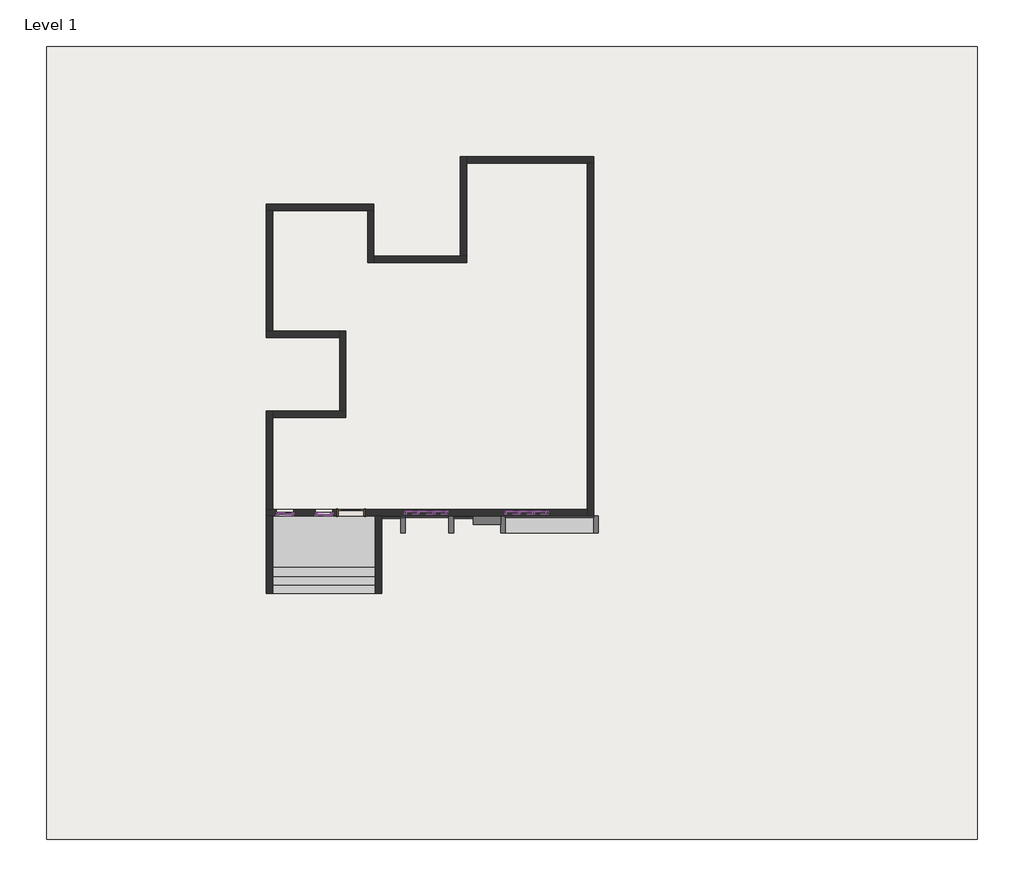
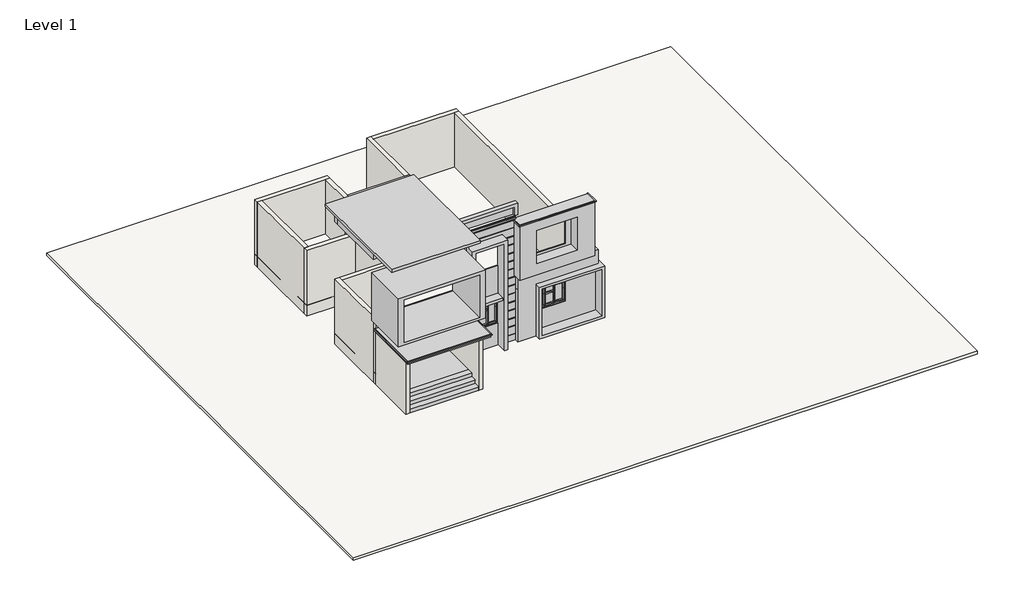
# One storey: 62 members, 18 plates, 14 walls, 2 slabs, 1 door, 1 proxy.
"""IFC4 building model written with IfcOpenShell, lengths in millimetres."""

from ifc_helpers import new_model, si_unit, frame, origin, origin_with_axes, place, context, project, spatial, polyline, outline, extrude, faceted_brep, transform, mapped, element, save
from components import generic_models_1_generic_models_1_556d1784, door_3b97b8e7, member_86d06fe4, member_323df77c, member_47bfaf8a, member_dffdf235, member_fd92426f, member_3709dd30, member_9ab3e039, member_2ebf4a73, member_ca359333, member_75d1e245, member_ffcd2ccf, member_b70ee1cc, member_3c3dc66a, member_dc106669, member_6428e230, member_5ae8a700, member_718fe5d9, member_bc7dbe04, member_90750a43, member_b2812fca, member_7fd687a9, member_26d576e8, member_fb4dac25, system_panel_glazed_c43f0a09, system_panel_glazed_07c93182, system_panel_glazed_e6031cb5, system_panel_glazed_9dd6121d, system_panel_glazed_f9f57b5d, system_panel_glazed_080879d4, system_panel_glazed_1c8147a1, system_panel_glazed_d072c6ac, system_panel_glazed_43ba880c, system_panel_glazed_00dbc574

model = new_model("IFC4")

# Units and contexts
model_context = context("Model", 3, world=origin())
ifc_project = project(units=[si_unit("LENGTHUNIT", "METRE", prefix="MILLI")], contexts=[model_context])

# Site, building, storey
site = spatial("IfcSite", under=ifc_project)
building = spatial("IfcBuilding", under=site)
storey = spatial("IfcBuildingStorey", under=building, Name="Level 1", Elevation=0.0)

# Proxy
placement = place(None, origin())
generic_models_1_generic_models_1_shape = generic_models_1_generic_models_1_556d1784(model_context)
element("IfcBuildingElementProxy", 1, Name="Generic Models 1 : Generic Models 1", ObjectType="Generic Models 1 : Generic Models 1", at=placement, inside=storey, context=model_context, shape_type="MappedRepresentation", body=[
    mapped(generic_models_1_generic_models_1_shape, transform((0.0, 0.0, 0.0), x_axis=(1.0, 0.0, 0.0), y_axis=(0.0, 1.0, 0.0), z_axis=(0.0, 0.0, 1.0))),
])

# Door
door_shape = door_3b97b8e7(model_context)
element("IfcDoor", 2, ObjectType="Door-Interior-Single-1_Panel-Wood : 36\" x 84\"", at=placement, inside=storey, context=model_context, shape_type="MappedRepresentation", body=[
    mapped(door_shape, transform((-9162.1679297, 32.0946292, 609.6), x_axis=(1.0, 0.0, 0.0), y_axis=(0.0, 1.0, 0.0), z_axis=(0.0, 0.0, 1.0))),
])

# Members
member_shape = member_86d06fe4(model_context)
element("IfcMember", 3, ObjectType="Rectangular Mullion : 2.5\" x 5\" rectangular", at=placement, inside=storey, context=model_context, shape_type="MappedRepresentation", body=[
    mapped(member_shape, transform((-10360.5848984, -34.5803708, 2743.2), x_axis=(0.0, 0.0, 1.0), y_axis=(0.0, 1.0, 0.0), z_axis=(-1.0, 0.0, 0.0))),
])
element("IfcMember", 4, ObjectType="Rectangular Mullion : 2.5\" x 5\" rectangular", at=placement, inside=storey, context=model_context, shape_type="MappedRepresentation", body=[
    mapped(member_shape, transform((-11257.6679297, -34.5803708, 2743.2), x_axis=(0.0, 0.0, 1.0), y_axis=(0.0, -1.0, 0.0), z_axis=(1.0, 0.0, 0.0))),
])
element("IfcMember", 5, ObjectType="Rectangular Mullion : 2.5\" x 5\" rectangular", at=placement, inside=storey, context=model_context, shape_type="MappedRepresentation", body=[
    mapped(member_shape, transform((-9877.9848984, -34.5803708, 914.4), x_axis=(0.0, 0.0, -1.0), y_axis=(0.0, 1.0, 0.0), z_axis=(1.0, 0.0, 0.0))),
])
element("IfcMember", 6, ObjectType="Rectangular Mullion : 2.5\" x 5\" rectangular", at=placement, inside=storey, context=model_context, shape_type="MappedRepresentation", body=[
    mapped(member_shape, transform((-11740.2679297, -34.5803708, 914.4), x_axis=(0.0, 0.0, -1.0), y_axis=(0.0, -1.0, 0.0), z_axis=(-1.0, 0.0, 0.0))),
])
member_2_shape = member_323df77c(model_context)
element("IfcMember", 7, ObjectType="Rectangular Mullion : 2.5\" x 5\" rectangular", at=placement, inside=storey, context=model_context, shape_type="MappedRepresentation", body=[
    mapped(member_2_shape, transform((-10360.5848984, -34.5803708, 2133.6), x_axis=(0.0, 0.0, 1.0), y_axis=(0.0, 1.0, 0.0), z_axis=(-1.0, 0.0, 0.0))),
])
element("IfcMember", 8, ObjectType="Rectangular Mullion : 2.5\" x 5\" rectangular", at=placement, inside=storey, context=model_context, shape_type="MappedRepresentation", body=[
    mapped(member_2_shape, transform((-10360.5848984, -34.5803708, 1524.0), x_axis=(0.0, 0.0, 1.0), y_axis=(0.0, 1.0, 0.0), z_axis=(-1.0, 0.0, 0.0))),
])
element("IfcMember", 9, ObjectType="Rectangular Mullion : 2.5\" x 5\" rectangular", at=placement, inside=storey, context=model_context, shape_type="MappedRepresentation", body=[
    mapped(member_2_shape, transform((-11257.6679297, -34.5803708, 2133.6), x_axis=(0.0, 0.0, 1.0), y_axis=(0.0, -1.0, 0.0), z_axis=(1.0, 0.0, 0.0))),
])
element("IfcMember", 10, ObjectType="Rectangular Mullion : 2.5\" x 5\" rectangular", at=placement, inside=storey, context=model_context, shape_type="MappedRepresentation", body=[
    mapped(member_2_shape, transform((-11257.6679297, -34.5803708, 1524.0), x_axis=(0.0, 0.0, 1.0), y_axis=(0.0, -1.0, 0.0), z_axis=(1.0, 0.0, 0.0))),
])
member_3_shape = member_47bfaf8a(model_context)
element("IfcMember", 11, ObjectType="Rectangular Mullion : 2.5\" x 5\" rectangular", at=placement, inside=storey, context=model_context, shape_type="MappedRepresentation", body=[
    mapped(member_3_shape, transform((-9814.4848984, -34.5803708, 2743.2), x_axis=(1.0, 0.0, 0.0), y_axis=(0.0, 1.0, 0.0), z_axis=(0.0, 0.0, 1.0))),
])
element("IfcMember", 12, ObjectType="Rectangular Mullion : 2.5\" x 5\" rectangular", at=placement, inside=storey, context=model_context, shape_type="MappedRepresentation", body=[
    mapped(member_3_shape, transform((-11803.7679297, -34.5803708, 2743.2), x_axis=(-1.0, 0.0, 0.0), y_axis=(0.0, -1.0, 0.0), z_axis=(0.0, 0.0, 1.0))),
])
element("IfcMember", 13, ObjectType="Rectangular Mullion : 2.5\" x 5\" rectangular", at=placement, inside=storey, context=model_context, shape_type="MappedRepresentation", body=[
    mapped(member_3_shape, transform((-10424.0848984, -34.5803708, 914.4), x_axis=(-1.0, 0.0, 0.0), y_axis=(0.0, 1.0, 0.0), z_axis=(0.0, 0.0, -1.0))),
])
element("IfcMember", 14, ObjectType="Rectangular Mullion : 2.5\" x 5\" rectangular", at=placement, inside=storey, context=model_context, shape_type="MappedRepresentation", body=[
    mapped(member_3_shape, transform((-11194.1679297, -34.5803708, 914.4), x_axis=(1.0, 0.0, 0.0), y_axis=(0.0, -1.0, 0.0), z_axis=(0.0, 0.0, -1.0))),
])
element("IfcMember", 15, ObjectType="Rectangular Mullion : 2.5\" x 5\" rectangular", at=placement, inside=storey, context=model_context, shape_type="MappedRepresentation", body=[
    mapped(member_3_shape, transform((-10424.0848984, -34.5803708, 2133.6), x_axis=(-1.0, 0.0, 0.0), y_axis=(0.0, 1.0, 0.0), z_axis=(0.0, 0.0, -1.0))),
])
element("IfcMember", 16, ObjectType="Rectangular Mullion : 2.5\" x 5\" rectangular", at=placement, inside=storey, context=model_context, shape_type="MappedRepresentation", body=[
    mapped(member_3_shape, transform((-11194.1679297, -34.5803708, 2133.6), x_axis=(1.0, 0.0, 0.0), y_axis=(0.0, -1.0, 0.0), z_axis=(0.0, 0.0, -1.0))),
])
element("IfcMember", 17, ObjectType="Rectangular Mullion : 2.5\" x 5\" rectangular", at=placement, inside=storey, context=model_context, shape_type="MappedRepresentation", body=[
    mapped(member_3_shape, transform((-10424.0848984, -34.5803708, 1524.0), x_axis=(-1.0, 0.0, 0.0), y_axis=(0.0, 1.0, 0.0), z_axis=(0.0, 0.0, -1.0))),
])
element("IfcMember", 18, ObjectType="Rectangular Mullion : 2.5\" x 5\" rectangular", at=placement, inside=storey, context=model_context, shape_type="MappedRepresentation", body=[
    mapped(member_3_shape, transform((-11194.1679297, -34.5803708, 1524.0), x_axis=(1.0, 0.0, 0.0), y_axis=(0.0, -1.0, 0.0), z_axis=(0.0, 0.0, -1.0))),
])
element("IfcMember", 19, ObjectType="Rectangular Mullion : 2.5\" x 5\" rectangular", at=placement, inside=storey, context=model_context, shape_type="MappedRepresentation", body=[
    mapped(member_3_shape, transform((-9814.4848984, -34.5803708, 2133.6), x_axis=(1.0, 0.0, 0.0), y_axis=(0.0, 1.0, 0.0), z_axis=(0.0, 0.0, 1.0))),
])
element("IfcMember", 20, ObjectType="Rectangular Mullion : 2.5\" x 5\" rectangular", at=placement, inside=storey, context=model_context, shape_type="MappedRepresentation", body=[
    mapped(member_3_shape, transform((-11803.7679297, -34.5803708, 2133.6), x_axis=(-1.0, 0.0, 0.0), y_axis=(0.0, -1.0, 0.0), z_axis=(0.0, 0.0, 1.0))),
])
element("IfcMember", 21, ObjectType="Rectangular Mullion : 2.5\" x 5\" rectangular", at=placement, inside=storey, context=model_context, shape_type="MappedRepresentation", body=[
    mapped(member_3_shape, transform((-9814.4848984, -34.5803708, 1524.0), x_axis=(1.0, 0.0, 0.0), y_axis=(0.0, 1.0, 0.0), z_axis=(0.0, 0.0, 1.0))),
])
element("IfcMember", 22, ObjectType="Rectangular Mullion : 2.5\" x 5\" rectangular", at=placement, inside=storey, context=model_context, shape_type="MappedRepresentation", body=[
    mapped(member_3_shape, transform((-11803.7679297, -34.5803708, 1524.0), x_axis=(-1.0, 0.0, 0.0), y_axis=(0.0, -1.0, 0.0), z_axis=(0.0, 0.0, 1.0))),
])
member_4_shape = member_dffdf235(model_context)
element("IfcMember", 23, ObjectType="Rectangular Mullion : 2.5\" x 5\" rectangular", at=placement, inside=storey, context=model_context, shape_type="MappedRepresentation", body=[
    mapped(member_4_shape, transform((-5796.6679297, 28.9196292, 2743.2), x_axis=(0.0, 0.0, 1.0), y_axis=(0.0, -1.0, 0.0), z_axis=(1.0, 0.0, 0.0))),
])
element("IfcMember", 24, ObjectType="Rectangular Mullion : 2.5\" x 5\" rectangular", at=placement, inside=storey, context=model_context, shape_type="MappedRepresentation", body=[
    mapped(member_4_shape, transform((-6806.3179297, 28.9196292, 2743.2), x_axis=(0.0, 0.0, 1.0), y_axis=(0.0, -1.0, 0.0), z_axis=(1.0, 0.0, 0.0))),
])
element("IfcMember", 25, ObjectType="Rectangular Mullion : 2.5\" x 5\" rectangular", at=placement, inside=storey, context=model_context, shape_type="MappedRepresentation", body=[
    mapped(member_4_shape, transform((-7193.6679297, 28.9196292, 1219.2), x_axis=(0.0, 0.0, -1.0), y_axis=(0.0, -1.0, 0.0), z_axis=(-1.0, 0.0, 0.0))),
])
element("IfcMember", 26, ObjectType="Rectangular Mullion : 2.5\" x 5\" rectangular", at=placement, inside=storey, context=model_context, shape_type="MappedRepresentation", body=[
    mapped(member_4_shape, transform((-6184.0179297, 28.9196292, 1219.2), x_axis=(0.0, 0.0, -1.0), y_axis=(0.0, -1.0, 0.0), z_axis=(-1.0, 0.0, 0.0))),
])
member_5_shape = member_fd92426f(model_context)
element("IfcMember", 27, ObjectType="Rectangular Mullion : 2.5\" x 5\" rectangular", at=placement, inside=storey, context=model_context, shape_type="MappedRepresentation", body=[
    mapped(member_5_shape, transform((-6774.5679297, 28.9196292, 1219.2), x_axis=(1.0, 0.0, 0.0), y_axis=(0.0, -1.0, 0.0), z_axis=(0.0, 0.0, -1.0))),
])
element("IfcMember", 28, ObjectType="Rectangular Mullion : 2.5\" x 5\" rectangular", at=placement, inside=storey, context=model_context, shape_type="MappedRepresentation", body=[
    mapped(member_5_shape, transform((-6215.7679297, 28.9196292, 1219.2), x_axis=(1.0, 0.0, 0.0), y_axis=(0.0, -1.0, 0.0), z_axis=(0.0, 0.0, -1.0))),
])
member_6_shape = member_3709dd30(model_context)
element("IfcMember", 29, ObjectType="Rectangular Mullion : 2.5\" x 5\" rectangular", at=placement, inside=storey, context=model_context, shape_type="MappedRepresentation", body=[
    mapped(member_6_shape, transform((-6806.3179297, 28.9196292, 2387.6), x_axis=(0.0, 0.0, 1.0), y_axis=(0.0, -1.0, 0.0), z_axis=(1.0, 0.0, 0.0))),
])
element("IfcMember", 30, ObjectType="Rectangular Mullion : 2.5\" x 5\" rectangular", at=placement, inside=storey, context=model_context, shape_type="MappedRepresentation", body=[
    mapped(member_6_shape, transform((-5796.6679297, 28.9196292, 2387.6), x_axis=(0.0, 0.0, 1.0), y_axis=(0.0, -1.0, 0.0), z_axis=(1.0, 0.0, 0.0))),
])
member_7_shape = member_9ab3e039(model_context)
element("IfcMember", 31, ObjectType="Rectangular Mullion : 2.5\" x 5\" rectangular", at=placement, inside=storey, context=model_context, shape_type="MappedRepresentation", body=[
    mapped(member_7_shape, transform((-6247.5179297, 28.9196292, 2082.8), x_axis=(0.0, 0.0, 1.0), y_axis=(0.0, -1.0, 0.0), z_axis=(1.0, 0.0, 0.0))),
])
member_8_shape = member_2ebf4a73(model_context)
element("IfcMember", 32, ObjectType="Rectangular Mullion : 2.5\" x 5\" rectangular", at=placement, inside=storey, context=model_context, shape_type="MappedRepresentation", body=[
    mapped(member_8_shape, transform((-6742.8179297, 28.9196292, 1219.2), x_axis=(0.0, 0.0, -1.0), y_axis=(0.0, -1.0, 0.0), z_axis=(-1.0, 0.0, 0.0))),
])
element("IfcMember", 33, ObjectType="Rectangular Mullion : 2.5\" x 5\" rectangular", at=placement, inside=storey, context=model_context, shape_type="MappedRepresentation", body=[
    mapped(member_8_shape, transform((-6247.5179297, 28.9196292, 2743.2), x_axis=(0.0, 0.0, 1.0), y_axis=(0.0, -1.0, 0.0), z_axis=(1.0, 0.0, 0.0))),
])
member_9_shape = member_ca359333(model_context)
element("IfcMember", 34, ObjectType="Rectangular Mullion : 2.5\" x 5\" rectangular", at=placement, inside=storey, context=model_context, shape_type="MappedRepresentation", body=[
    mapped(member_9_shape, transform((-6774.5679297, 28.9196292, 2387.6), x_axis=(1.0, 0.0, 0.0), y_axis=(0.0, -1.0, 0.0), z_axis=(0.0, 0.0, -1.0))),
])
element("IfcMember", 35, ObjectType="Rectangular Mullion : 2.5\" x 5\" rectangular", at=placement, inside=storey, context=model_context, shape_type="MappedRepresentation", body=[
    mapped(member_9_shape, transform((-6215.7679297, 28.9196292, 2387.6), x_axis=(1.0, 0.0, 0.0), y_axis=(0.0, -1.0, 0.0), z_axis=(0.0, 0.0, -1.0))),
])
member_10_shape = member_75d1e245(model_context)
element("IfcMember", 36, ObjectType="Rectangular Mullion : 2.5\" x 5\" rectangular", at=placement, inside=storey, context=model_context, shape_type="MappedRepresentation", body=[
    mapped(member_10_shape, transform((-6774.5679297, 28.9196292, 2082.8), x_axis=(1.0, 0.0, 0.0), y_axis=(0.0, -1.0, 0.0), z_axis=(0.0, 0.0, -1.0))),
])
element("IfcMember", 37, ObjectType="Rectangular Mullion : 2.5\" x 5\" rectangular", at=placement, inside=storey, context=model_context, shape_type="MappedRepresentation", body=[
    mapped(member_10_shape, transform((-6215.7679297, 28.9196292, 2082.8), x_axis=(1.0, 0.0, 0.0), y_axis=(0.0, -1.0, 0.0), z_axis=(0.0, 0.0, -1.0))),
])
member_11_shape = member_ffcd2ccf(model_context)
element("IfcMember", 38, ObjectType="Rectangular Mullion : 2.5\" x 5\" rectangular", at=placement, inside=storey, context=model_context, shape_type="MappedRepresentation", body=[
    mapped(member_11_shape, transform((-7257.1679297, 28.9196292, 2743.2), x_axis=(-1.0, 0.0, 0.0), y_axis=(0.0, -1.0, 0.0), z_axis=(0.0, 0.0, 1.0))),
])
member_12_shape = member_b70ee1cc(model_context)
element("IfcMember", 39, ObjectType="Rectangular Mullion : 2.5\" x 5\" rectangular", at=placement, inside=storey, context=model_context, shape_type="MappedRepresentation", body=[
    mapped(member_12_shape, transform((-5733.1679297, 28.9196292, 1219.2), x_axis=(1.0, 0.0, 0.0), y_axis=(0.0, -1.0, 0.0), z_axis=(0.0, 0.0, -1.0))),
])
element("IfcMember", 40, ObjectType="Rectangular Mullion : 2.5\" x 5\" rectangular", at=placement, inside=storey, context=model_context, shape_type="MappedRepresentation", body=[
    mapped(member_11_shape, transform((-5733.1679297, 28.9196292, 2387.6), x_axis=(1.0, 0.0, 0.0), y_axis=(0.0, -1.0, 0.0), z_axis=(0.0, 0.0, -1.0))),
])
member_13_shape = member_3c3dc66a(model_context)
element("IfcMember", 41, ObjectType="Rectangular Mullion : 2.5\" x 5\" rectangular", at=placement, inside=storey, context=model_context, shape_type="MappedRepresentation", body=[
    mapped(member_13_shape, transform((-5733.1679297, 28.9196292, 2082.8), x_axis=(1.0, 0.0, 0.0), y_axis=(0.0, -1.0, 0.0), z_axis=(0.0, 0.0, -1.0))),
])
element("IfcMember", 42, ObjectType="Rectangular Mullion : 2.5\" x 5\" rectangular", at=placement, inside=storey, context=model_context, shape_type="MappedRepresentation", body=[
    mapped(member_13_shape, transform((-7257.1679297, 28.9196292, 2387.6), x_axis=(-1.0, 0.0, 0.0), y_axis=(0.0, -1.0, 0.0), z_axis=(0.0, 0.0, 1.0))),
])
element("IfcMember", 43, ObjectType="Rectangular Mullion : 2.5\" x 5\" rectangular", at=placement, inside=storey, context=model_context, shape_type="MappedRepresentation", body=[
    mapped(member_12_shape, transform((-7257.1679297, 28.9196292, 2082.8), x_axis=(-1.0, 0.0, 0.0), y_axis=(0.0, -1.0, 0.0), z_axis=(0.0, 0.0, 1.0))),
])
member_14_shape = member_dc106669(model_context)
element("IfcMember", 44, ObjectType="Rectangular Mullion : 2.5\" x 5\" rectangular", at=placement, inside=storey, context=model_context, shape_type="MappedRepresentation", body=[
    mapped(member_14_shape, transform((-2253.3679297, 28.9196292, 2743.2), x_axis=(0.0, 0.0, 1.0), y_axis=(0.0, -1.0, 0.0), z_axis=(1.0, 0.0, 0.0))),
])
element("IfcMember", 45, ObjectType="Rectangular Mullion : 2.5\" x 5\" rectangular", at=placement, inside=storey, context=model_context, shape_type="MappedRepresentation", body=[
    mapped(member_14_shape, transform((-3237.6179297, 28.9196292, 2743.2), x_axis=(0.0, 0.0, 1.0), y_axis=(0.0, -1.0, 0.0), z_axis=(1.0, 0.0, 0.0))),
])
element("IfcMember", 46, ObjectType="Rectangular Mullion : 2.5\" x 5\" rectangular", at=placement, inside=storey, context=model_context, shape_type="MappedRepresentation", body=[
    mapped(member_14_shape, transform((-3650.3679297, 28.9196292, 1219.2), x_axis=(0.0, 0.0, -1.0), y_axis=(0.0, -1.0, 0.0), z_axis=(-1.0, 0.0, 0.0))),
])
element("IfcMember", 47, ObjectType="Rectangular Mullion : 2.5\" x 5\" rectangular", at=placement, inside=storey, context=model_context, shape_type="MappedRepresentation", body=[
    mapped(member_14_shape, transform((-2666.1179297, 28.9196292, 1219.2), x_axis=(0.0, 0.0, -1.0), y_axis=(0.0, -1.0, 0.0), z_axis=(-1.0, 0.0, 0.0))),
])
member_15_shape = member_6428e230(model_context)
element("IfcMember", 48, ObjectType="Rectangular Mullion : 2.5\" x 5\" rectangular", at=placement, inside=storey, context=model_context, shape_type="MappedRepresentation", body=[
    mapped(member_15_shape, transform((-3205.8679297, 28.9196292, 1219.2), x_axis=(1.0, 0.0, 0.0), y_axis=(0.0, -1.0, 0.0), z_axis=(0.0, 0.0, -1.0))),
])
element("IfcMember", 49, ObjectType="Rectangular Mullion : 2.5\" x 5\" rectangular", at=placement, inside=storey, context=model_context, shape_type="MappedRepresentation", body=[
    mapped(member_15_shape, transform((-2697.8679297, 28.9196292, 1219.2), x_axis=(1.0, 0.0, 0.0), y_axis=(0.0, -1.0, 0.0), z_axis=(0.0, 0.0, -1.0))),
])
member_16_shape = member_5ae8a700(model_context)
element("IfcMember", 50, ObjectType="Rectangular Mullion : 2.5\" x 5\" rectangular", at=placement, inside=storey, context=model_context, shape_type="MappedRepresentation", body=[
    mapped(member_16_shape, transform((-3237.6179297, 28.9196292, 2235.2), x_axis=(0.0, 0.0, 1.0), y_axis=(0.0, -1.0, 0.0), z_axis=(1.0, 0.0, 0.0))),
])
element("IfcMember", 51, ObjectType="Rectangular Mullion : 2.5\" x 5\" rectangular", at=placement, inside=storey, context=model_context, shape_type="MappedRepresentation", body=[
    mapped(member_16_shape, transform((-2253.3679297, 28.9196292, 2235.2), x_axis=(0.0, 0.0, 1.0), y_axis=(0.0, -1.0, 0.0), z_axis=(1.0, 0.0, 0.0))),
])
member_17_shape = member_718fe5d9(model_context)
element("IfcMember", 52, ObjectType="Rectangular Mullion : 2.5\" x 5\" rectangular", at=placement, inside=storey, context=model_context, shape_type="MappedRepresentation", body=[
    mapped(member_17_shape, transform((-2729.6179297, 28.9196292, 1896.5333333), x_axis=(0.0, 0.0, 1.0), y_axis=(0.0, -1.0, 0.0), z_axis=(1.0, 0.0, 0.0))),
])
member_18_shape = member_bc7dbe04(model_context)
element("IfcMember", 53, ObjectType="Rectangular Mullion : 2.5\" x 5\" rectangular", at=placement, inside=storey, context=model_context, shape_type="MappedRepresentation", body=[
    mapped(member_18_shape, transform((-3174.1179297, 28.9196292, 1219.2), x_axis=(0.0, 0.0, -1.0), y_axis=(0.0, -1.0, 0.0), z_axis=(-1.0, 0.0, 0.0))),
])
element("IfcMember", 54, ObjectType="Rectangular Mullion : 2.5\" x 5\" rectangular", at=placement, inside=storey, context=model_context, shape_type="MappedRepresentation", body=[
    mapped(member_18_shape, transform((-2729.6179297, 28.9196292, 2743.2), x_axis=(0.0, 0.0, 1.0), y_axis=(0.0, -1.0, 0.0), z_axis=(1.0, 0.0, 0.0))),
])
member_19_shape = member_90750a43(model_context)
element("IfcMember", 55, ObjectType="Rectangular Mullion : 2.5\" x 5\" rectangular", at=placement, inside=storey, context=model_context, shape_type="MappedRepresentation", body=[
    mapped(member_19_shape, transform((-3205.8679297, 28.9196292, 2235.2), x_axis=(1.0, 0.0, 0.0), y_axis=(0.0, -1.0, 0.0), z_axis=(0.0, 0.0, -1.0))),
])
element("IfcMember", 56, ObjectType="Rectangular Mullion : 2.5\" x 5\" rectangular", at=placement, inside=storey, context=model_context, shape_type="MappedRepresentation", body=[
    mapped(member_19_shape, transform((-2697.8679297, 28.9196292, 2235.2), x_axis=(1.0, 0.0, 0.0), y_axis=(0.0, -1.0, 0.0), z_axis=(0.0, 0.0, -1.0))),
])
member_20_shape = member_b2812fca(model_context)
element("IfcMember", 57, ObjectType="Rectangular Mullion : 2.5\" x 5\" rectangular", at=placement, inside=storey, context=model_context, shape_type="MappedRepresentation", body=[
    mapped(member_20_shape, transform((-3205.8679297, 28.9196292, 1896.5333333), x_axis=(1.0, 0.0, 0.0), y_axis=(0.0, -1.0, 0.0), z_axis=(0.0, 0.0, -1.0))),
])
element("IfcMember", 58, ObjectType="Rectangular Mullion : 2.5\" x 5\" rectangular", at=placement, inside=storey, context=model_context, shape_type="MappedRepresentation", body=[
    mapped(member_20_shape, transform((-2697.8679297, 28.9196292, 1896.5333333), x_axis=(1.0, 0.0, 0.0), y_axis=(0.0, -1.0, 0.0), z_axis=(0.0, 0.0, -1.0))),
])
member_21_shape = member_7fd687a9(model_context)
element("IfcMember", 59, ObjectType="Rectangular Mullion : 2.5\" x 5\" rectangular", at=placement, inside=storey, context=model_context, shape_type="MappedRepresentation", body=[
    mapped(member_21_shape, transform((-3713.8679297, 28.9196292, 2743.2), x_axis=(-1.0, 0.0, 0.0), y_axis=(0.0, -1.0, 0.0), z_axis=(0.0, 0.0, 1.0))),
])
member_22_shape = member_26d576e8(model_context)
element("IfcMember", 60, ObjectType="Rectangular Mullion : 2.5\" x 5\" rectangular", at=placement, inside=storey, context=model_context, shape_type="MappedRepresentation", body=[
    mapped(member_22_shape, transform((-2189.8679297, 28.9196292, 1219.2), x_axis=(1.0, 0.0, 0.0), y_axis=(0.0, -1.0, 0.0), z_axis=(0.0, 0.0, -1.0))),
])
element("IfcMember", 61, ObjectType="Rectangular Mullion : 2.5\" x 5\" rectangular", at=placement, inside=storey, context=model_context, shape_type="MappedRepresentation", body=[
    mapped(member_21_shape, transform((-2189.8679297, 28.9196292, 2235.2), x_axis=(1.0, 0.0, 0.0), y_axis=(0.0, -1.0, 0.0), z_axis=(0.0, 0.0, -1.0))),
])
member_23_shape = member_fb4dac25(model_context)
element("IfcMember", 62, ObjectType="Rectangular Mullion : 2.5\" x 5\" rectangular", at=placement, inside=storey, context=model_context, shape_type="MappedRepresentation", body=[
    mapped(member_23_shape, transform((-2189.8679297, 28.9196292, 1896.5333333), x_axis=(1.0, 0.0, 0.0), y_axis=(0.0, -1.0, 0.0), z_axis=(0.0, 0.0, -1.0))),
])
element("IfcMember", 63, ObjectType="Rectangular Mullion : 2.5\" x 5\" rectangular", at=placement, inside=storey, context=model_context, shape_type="MappedRepresentation", body=[
    mapped(member_23_shape, transform((-3713.8679297, 28.9196292, 2235.2), x_axis=(-1.0, 0.0, 0.0), y_axis=(0.0, -1.0, 0.0), z_axis=(0.0, 0.0, 1.0))),
])
element("IfcMember", 64, ObjectType="Rectangular Mullion : 2.5\" x 5\" rectangular", at=placement, inside=storey, context=model_context, shape_type="MappedRepresentation", body=[
    mapped(member_22_shape, transform((-3713.8679297, 28.9196292, 1896.5333333), x_axis=(-1.0, 0.0, 0.0), y_axis=(0.0, -1.0, 0.0), z_axis=(0.0, 0.0, 1.0))),
])

# Plates
system_panel_glazed_shape = system_panel_glazed_c43f0a09(model_context)
element("IfcPlate", 65, ObjectType="System Panel : Glazed", at=placement, inside=storey, context=model_context, shape_type="MappedRepresentation", body=[
    mapped(system_panel_glazed_shape, transform((-10119.2848984, -34.5803708, 977.9), x_axis=(-1.0, 0.0, 0.0), y_axis=(0.0, -1.0, 0.0), z_axis=(0.0, 0.0, 1.0))),
])
element("IfcPlate", 66, ObjectType="System Panel : Glazed", at=placement, inside=storey, context=model_context, shape_type="MappedRepresentation", body=[
    mapped(system_panel_glazed_shape, transform((-11498.9679297, -34.5803708, 977.9), x_axis=(1.0, 0.0, 0.0), y_axis=(0.0, 1.0, 0.0), z_axis=(0.0, 0.0, 1.0))),
])
element("IfcPlate", 67, ObjectType="System Panel : Glazed", at=placement, inside=storey, context=model_context, shape_type="MappedRepresentation", body=[
    mapped(system_panel_glazed_shape, transform((-11498.9679297, -34.5803708, 2165.35), x_axis=(1.0, 0.0, 0.0), y_axis=(0.0, 1.0, 0.0), z_axis=(0.0, 0.0, 1.0))),
])
element("IfcPlate", 68, ObjectType="System Panel : Glazed", at=placement, inside=storey, context=model_context, shape_type="MappedRepresentation", body=[
    mapped(system_panel_glazed_shape, transform((-10119.2848984, -34.5803708, 2165.35), x_axis=(-1.0, 0.0, 0.0), y_axis=(0.0, -1.0, 0.0), z_axis=(0.0, 0.0, 1.0))),
])
system_panel_glazed_2_shape = system_panel_glazed_07c93182(model_context)
element("IfcPlate", 69, ObjectType="System Panel : Glazed", at=placement, inside=storey, context=model_context, shape_type="MappedRepresentation", body=[
    mapped(system_panel_glazed_2_shape, transform((-11498.9679297, -34.5803708, 1555.75), x_axis=(1.0, 0.0, 0.0), y_axis=(0.0, 1.0, 0.0), z_axis=(0.0, 0.0, 1.0))),
])
element("IfcPlate", 70, ObjectType="System Panel : Glazed", at=placement, inside=storey, context=model_context, shape_type="MappedRepresentation", body=[
    mapped(system_panel_glazed_2_shape, transform((-10119.2848984, -34.5803708, 1555.75), x_axis=(-1.0, 0.0, 0.0), y_axis=(0.0, -1.0, 0.0), z_axis=(0.0, 0.0, 1.0))),
])
system_panel_glazed_3_shape = system_panel_glazed_e6031cb5(model_context)
element("IfcPlate", 71, ObjectType="System Panel : Glazed", at=placement, inside=storey, context=model_context, shape_type="MappedRepresentation", body=[
    mapped(system_panel_glazed_3_shape, transform((-6999.9929297, 28.9196292, 1282.7), x_axis=(1.0, 0.0, 0.0), y_axis=(0.0, 1.0, 0.0), z_axis=(0.0, 0.0, 1.0))),
])
element("IfcPlate", 72, ObjectType="System Panel : Glazed", at=placement, inside=storey, context=model_context, shape_type="MappedRepresentation", body=[
    mapped(system_panel_glazed_3_shape, transform((-5990.3429297, 28.9196292, 1282.7), x_axis=(1.0, 0.0, 0.0), y_axis=(0.0, 1.0, 0.0), z_axis=(0.0, 0.0, 1.0))),
])
system_panel_glazed_4_shape = system_panel_glazed_9dd6121d(model_context)
element("IfcPlate", 73, ObjectType="System Panel : Glazed", at=placement, inside=storey, context=model_context, shape_type="MappedRepresentation", body=[
    mapped(system_panel_glazed_4_shape, transform((-6495.1679297, 28.9196292, 1282.7), x_axis=(1.0, 0.0, 0.0), y_axis=(0.0, 1.0, 0.0), z_axis=(0.0, 0.0, 1.0))),
])
system_panel_glazed_5_shape = system_panel_glazed_f9f57b5d(model_context)
element("IfcPlate", 74, ObjectType="System Panel : Glazed", at=placement, inside=storey, context=model_context, shape_type="MappedRepresentation", body=[
    mapped(system_panel_glazed_5_shape, transform((-6999.9929297, 28.9196292, 2419.35), x_axis=(1.0, 0.0, 0.0), y_axis=(0.0, 1.0, 0.0), z_axis=(0.0, 0.0, 1.0))),
])
element("IfcPlate", 75, ObjectType="System Panel : Glazed", at=placement, inside=storey, context=model_context, shape_type="MappedRepresentation", body=[
    mapped(system_panel_glazed_5_shape, transform((-5990.3429297, 28.9196292, 2419.35), x_axis=(1.0, 0.0, 0.0), y_axis=(0.0, 1.0, 0.0), z_axis=(0.0, 0.0, 1.0))),
])
system_panel_glazed_6_shape = system_panel_glazed_080879d4(model_context)
element("IfcPlate", 76, ObjectType="System Panel : Glazed", at=placement, inside=storey, context=model_context, shape_type="MappedRepresentation", body=[
    mapped(system_panel_glazed_6_shape, transform((-6495.1679297, 28.9196292, 2114.55), x_axis=(1.0, 0.0, 0.0), y_axis=(0.0, 1.0, 0.0), z_axis=(0.0, 0.0, 1.0))),
])
system_panel_glazed_7_shape = system_panel_glazed_1c8147a1(model_context)
element("IfcPlate", 77, ObjectType="System Panel : Glazed", at=placement, inside=storey, context=model_context, shape_type="MappedRepresentation", body=[
    mapped(system_panel_glazed_7_shape, transform((-3443.9929297, 28.9196292, 1282.7), x_axis=(1.0, 0.0, 0.0), y_axis=(0.0, 1.0, 0.0), z_axis=(0.0, 0.0, 1.0))),
])
element("IfcPlate", 78, ObjectType="System Panel : Glazed", at=placement, inside=storey, context=model_context, shape_type="MappedRepresentation", body=[
    mapped(system_panel_glazed_7_shape, transform((-2459.7429297, 28.9196292, 1282.7), x_axis=(1.0, 0.0, 0.0), y_axis=(0.0, 1.0, 0.0), z_axis=(0.0, 0.0, 1.0))),
])
system_panel_glazed_8_shape = system_panel_glazed_d072c6ac(model_context)
element("IfcPlate", 79, ObjectType="System Panel : Glazed", at=placement, inside=storey, context=model_context, shape_type="MappedRepresentation", body=[
    mapped(system_panel_glazed_8_shape, transform((-2951.8679297, 28.9196292, 1282.7), x_axis=(1.0, 0.0, 0.0), y_axis=(0.0, 1.0, 0.0), z_axis=(0.0, 0.0, 1.0))),
])
system_panel_glazed_9_shape = system_panel_glazed_43ba880c(model_context)
element("IfcPlate", 80, ObjectType="System Panel : Glazed", at=placement, inside=storey, context=model_context, shape_type="MappedRepresentation", body=[
    mapped(system_panel_glazed_9_shape, transform((-3443.9929297, 28.9196292, 2266.95), x_axis=(1.0, 0.0, 0.0), y_axis=(0.0, 1.0, 0.0), z_axis=(0.0, 0.0, 1.0))),
])
element("IfcPlate", 81, ObjectType="System Panel : Glazed", at=placement, inside=storey, context=model_context, shape_type="MappedRepresentation", body=[
    mapped(system_panel_glazed_9_shape, transform((-2459.7429297, 28.9196292, 2266.95), x_axis=(1.0, 0.0, 0.0), y_axis=(0.0, 1.0, 0.0), z_axis=(0.0, 0.0, 1.0))),
])
system_panel_glazed_10_shape = system_panel_glazed_00dbc574(model_context)
element("IfcPlate", 82, ObjectType="System Panel : Glazed", at=placement, inside=storey, context=model_context, shape_type="MappedRepresentation", body=[
    mapped(system_panel_glazed_10_shape, transform((-2951.8679297, 28.9196292, 1928.2833333), x_axis=(1.0, 0.0, 0.0), y_axis=(0.0, 1.0, 0.0), z_axis=(0.0, 0.0, 1.0))),
])

# Slabs
element("IfcSlab", 83, ObjectType="6\" floor", at=placement, inside=storey, context=model_context, shape_type="SweptSolid", body=[
    extrude(outline(polyline([(-12159.3679297, 10938.2196292), (-8349.3679297, 10938.2196292), (-8349.3679297, 9109.4196292), (-5301.3679297, 9109.4196292), (-5301.3679297, 12614.6196292), (-576.9679297, 12614.6196292), (-576.9679297, -85.3803708), (-12159.3679297, -85.3803708), (-12159.3679297, 3623.0196292), (-9568.5679297, 3623.0196292), (-9568.5679297, 6213.8196292), (-12159.3679297, 6213.8196292), (-12159.3679297, 10938.2196292)])), frame((0.0, 0.0, 457.2), z_axis=(0.0, 0.0, 1.0), x_axis=(1.0, 0.0, 0.0)), (0.0, 0.0, 1.0), 152.4),
])
element("IfcSlab", 84, ObjectType="6\" floor 2", at=placement, inside=storey, context=model_context, shape_type="SweptSolid", body=[
    extrude(outline(polyline([(12990.0083938, 16518.8927904), (12990.0083938, -11522.7072096), (-19928.3916062, -11522.7072096), (-19928.3916062, 16518.8927904), (12990.0083938, 16518.8927904)])), frame((0.0, 0.0, -152.4), z_axis=(0.0, 0.0, 1.0), x_axis=(1.0, 0.0, 0.0)), (0.0, 0.0, 1.0), 152.4),
])

# Walls
element("IfcWall", 85, ObjectType="9\" wall", at=placement, inside=storey, context=model_context, shape_type="Brep", body=[
    faceted_brep([(-12159.3679297, 10709.6196292, 0.0), (-11930.7679297, 10709.6196292, 0.0), (-8577.9679297, 10709.6196292, 0.0), (-8349.3679297, 10709.6196292, 0.0), (-8349.3679297, 10709.6196292, 3657.6), (-8577.9679297, 10709.6196292, 3657.6), (-11930.7679297, 10709.6196292, 3657.6), (-12159.3679297, 10709.6196292, 3657.6), (-12159.3679297, 10938.2196292, 0.0), (-12159.3679297, 10938.2196292, 3657.6), (-8349.3679297, 10938.2196292, 3657.6), (-8349.3679297, 10938.2196292, 0.0)], [[[0, 1, 2, 3, 4, 5, 6, 7]], [[8, 9, 10, 11]], [[3, 2, 1, 0, 8, 11]], [[7, 6, 5, 4, 10, 9]], [[4, 3, 11, 10]], [[0, 7, 9, 8]]]),
])
element("IfcWall", 86, ObjectType="9\" wall", at=placement, inside=storey, context=model_context, shape_type="Brep", body=[
    faceted_brep([(-8577.9679297, 10709.6196292, 0.0), (-8577.9679297, 8880.8196292, 0.0), (-8577.9679297, 8880.8196292, 3657.6), (-8577.9679297, 10709.6196292, 3657.6), (-8349.3679297, 10709.6196292, 0.0), (-8349.3679297, 10709.6196292, 3657.6), (-8349.3679297, 9109.4196292, 3657.6), (-8349.3679297, 8880.8196292, 3657.6), (-8349.3679297, 8880.8196292, 0.0), (-8349.3679297, 9109.4196292, 0.0)], [[[0, 1, 2, 3]], [[4, 5, 6, 7, 8, 9]], [[1, 0, 4, 9, 8]], [[3, 2, 7, 6, 5]], [[0, 3, 5, 4]], [[2, 1, 8, 7]]]),
])
element("IfcWall", 87, ObjectType="9\" wall", at=placement, inside=storey, context=model_context, shape_type="Brep", body=[
    faceted_brep([(-8349.3679297, 8880.8196292, 0.0), (-5072.7679297, 8880.8196292, 0.0), (-5072.7679297, 8880.8196292, 3657.6), (-8349.3679297, 8880.8196292, 3657.6), (-8349.3679297, 9109.4196292, 0.0), (-8349.3679297, 9109.4196292, 3657.6), (-5301.3679297, 9109.4196292, 3657.6), (-5072.7679297, 9109.4196292, 3657.6), (-5072.7679297, 9109.4196292, 0.0), (-5301.3679297, 9109.4196292, 0.0)], [[[0, 1, 2, 3]], [[4, 5, 6, 7, 8, 9]], [[1, 0, 4, 9, 8]], [[3, 2, 7, 6, 5]], [[0, 3, 5, 4]], [[2, 1, 8, 7]]]),
])
element("IfcWall", 88, ObjectType="9\" wall", at=placement, inside=storey, context=model_context, shape_type="Brep", body=[
    faceted_brep([(-5072.7679297, 9109.4196292, 0.0), (-5072.7679297, 12386.0196292, 0.0), (-5072.7679297, 12614.6196292, 0.0), (-5072.7679297, 12614.6196292, 3657.6), (-5072.7679297, 12386.0196292, 3657.6), (-5072.7679297, 9109.4196292, 3657.6), (-5301.3679297, 9109.4196292, 0.0), (-5301.3679297, 9109.4196292, 3657.6), (-5301.3679297, 12614.6196292, 3657.6), (-5301.3679297, 12614.6196292, 0.0)], [[[0, 1, 2, 3, 4, 5]], [[6, 7, 8, 9]], [[2, 1, 0, 6, 9]], [[5, 4, 3, 8, 7]], [[0, 5, 7, 6]], [[3, 2, 9, 8]]]),
])
element("IfcWall", 89, ObjectType="9\" wall", at=placement, inside=storey, context=model_context, shape_type="Brep", body=[
    faceted_brep([(-5072.7679297, 12386.0196292, 0.0), (-805.5679297, 12386.0196292, 0.0), (-576.9679297, 12386.0196292, 0.0), (-576.9679297, 12386.0196292, 3657.6), (-805.5679297, 12386.0196292, 3657.6), (-5072.7679297, 12386.0196292, 3657.6), (-5072.7679297, 12614.6196292, 0.0), (-5072.7679297, 12614.6196292, 3657.6), (-576.9679297, 12614.6196292, 3657.6), (-576.9679297, 12614.6196292, 0.0)], [[[0, 1, 2, 3, 4, 5]], [[6, 7, 8, 9]], [[2, 1, 0, 6, 9]], [[5, 4, 3, 8, 7]], [[0, 5, 7, 6]], [[3, 2, 9, 8]]]),
])
element("IfcWall", 90, ObjectType="9\" wall", at=placement, inside=storey, context=model_context, shape_type="Brep", body=[
    faceted_brep([(-805.5679297, 12386.0196292, 0.0), (-805.5679297, 143.2196292, 0.0), (-805.5679297, -85.3803708, 0.0), (-805.5679297, -85.3803708, 3657.6), (-805.5679297, 143.2196292, 3657.6), (-805.5679297, 12386.0196292, 3657.6), (-576.9679297, 12386.0196292, 0.0), (-576.9679297, 12386.0196292, 3657.6), (-576.9679297, -85.3803708, 3657.6), (-576.9679297, -85.3803708, 0.0)], [[[0, 1, 2, 3, 4, 5]], [[6, 7, 8, 9]], [[2, 1, 0, 6, 9]], [[5, 4, 3, 8, 7]], [[0, 5, 7, 6]], [[3, 2, 9, 8]]]),
])
element("IfcWall", 91, ObjectType="9\" wall", at=placement, inside=storey, context=model_context, shape_type="Brep", body=[
    faceted_brep([(-805.5679297, 143.2196292, 0.0), (-11930.7679297, 143.2196292, 0.0), (-12159.3679297, 143.2196292, 0.0), (-12159.3679297, 143.2196292, 3657.6), (-11930.7679297, 143.2196292, 3657.6), (-805.5679297, 143.2196292, 3657.6), (-8679.5679297, 143.2196292, 609.6), (-8679.5679297, 143.2196292, 2768.6), (-9644.7679297, 143.2196292, 2768.6), (-9644.7679297, 143.2196292, 609.6), (-11803.7679297, 143.2196292, 2743.2), (-11803.7679297, 143.2196292, 914.4), (-11194.1679297, 143.2196292, 914.4), (-11194.1679297, 143.2196292, 2743.2), (-9814.4848984, 143.2196292, 914.4), (-9814.4848984, 143.2196292, 2743.2), (-10424.0848984, 143.2196292, 2743.2), (-10424.0848984, 143.2196292, 914.4), (-7257.1679297, 143.2196292, 2743.2), (-7257.1679297, 143.2196292, 1219.2), (-5733.1679297, 143.2196292, 1219.2), (-5733.1679297, 143.2196292, 2743.2), (-3713.8679297, 143.2196292, 2743.2), (-3713.8679297, 143.2196292, 1219.2), (-2189.8679297, 143.2196292, 1219.2), (-2189.8679297, 143.2196292, 2743.2), (-12159.3679297, -85.3803708, 0.0), (-11930.7679297, -85.3803708, 0.0), (-8311.2679297, -85.3803708, 0.0), (-8082.6679297, -85.3803708, 0.0), (-805.5679297, -85.3803708, 0.0), (-805.5679297, -85.3803708, 3657.6), (-7879.4679297, -85.3803708, 3657.6), (-7981.0679297, -85.3803708, 3657.6), (-12095.8679297, -85.3803708, 3657.6), (-12159.3679297, -85.3803708, 3657.6), (-12159.3679297, -85.3803708, 2984.9208873), (-8679.5679297, -85.3803708, 2768.6), (-8679.5679297, -85.3803708, 609.6), (-9644.7679297, -85.3803708, 609.6), (-9644.7679297, -85.3803708, 2768.6), (-11803.7679297, -85.3803708, 914.4), (-11803.7679297, -85.3803708, 2743.2), (-11194.1679297, -85.3803708, 2743.2), (-11194.1679297, -85.3803708, 914.4), (-9814.4848984, -85.3803708, 2743.2), (-9814.4848984, -85.3803708, 914.4), (-10424.0848984, -85.3803708, 914.4), (-10424.0848984, -85.3803708, 2743.2), (-7257.1679297, -85.3803708, 1219.2), (-7257.1679297, -85.3803708, 2743.2), (-5733.1679297, -85.3803708, 2743.2), (-5733.1679297, -85.3803708, 1219.2), (-3713.8679297, -85.3803708, 1219.2), (-3713.8679297, -85.3803708, 2743.2), (-2189.8679297, -85.3803708, 2743.2), (-2189.8679297, -85.3803708, 1219.2)], [[[0, 1, 2, 3, 4, 5], [6, 7, 8, 9], [10, 11, 12, 13], [14, 15, 16, 17], [18, 19, 20, 21], [22, 23, 24, 25]], [[26, 27, 28, 29, 30, 31, 32, 33, 34, 35, 36], [37, 38, 39, 40], [41, 42, 43, 44], [45, 46, 47, 48], [49, 50, 51, 52], [53, 54, 55, 56]], [[2, 1, 0, 30, 29, 28, 27, 26]], [[5, 4, 3, 35, 34, 33, 32, 31]], [[6, 38, 37, 7]], [[7, 37, 40, 8]], [[39, 9, 8, 40]], [[38, 6, 9, 39]], [[41, 11, 10, 42]], [[42, 10, 13, 43]], [[43, 13, 12, 44]], [[11, 41, 44, 12]], [[45, 15, 14, 46]], [[15, 45, 48, 16]], [[16, 48, 47, 17]], [[46, 14, 17, 47]], [[0, 5, 31, 30]], [[2, 26, 36, 35, 3]], [[49, 19, 18, 50]], [[50, 18, 21, 51]], [[20, 52, 51, 21]], [[19, 49, 52, 20]], [[53, 23, 22, 54]], [[54, 22, 25, 55]], [[24, 56, 55, 25]], [[23, 53, 56, 24]]]),
])
element("IfcWall", 92, ObjectType="9\" wall", at=placement, inside=storey, context=model_context, shape_type="Brep", body=[
    faceted_brep([(-11930.7679297, 143.2196292, 3657.6), (-11930.7679297, 143.2196292, 0.0), (-11930.7679297, 3394.4196292, 0.0), (-11930.7679297, 3623.0196292, 0.0), (-11930.7679297, 3623.0196292, 3657.6), (-11930.7679297, 3394.4196292, 3657.6), (-12159.3679297, 143.2196292, 0.0), (-12159.3679297, 143.2196292, 3657.6), (-12159.3679297, 3623.0196292, 3657.6), (-12159.3679297, 3623.0196292, 0.0)], [[[0, 1, 2, 3, 4, 5]], [[6, 7, 8, 9]], [[3, 2, 1, 6, 9]], [[0, 5, 4, 8, 7]], [[4, 3, 9, 8]], [[0, 7, 6, 1]]]),
])
element("IfcWall", 93, ObjectType="9\" wall", at=placement, inside=storey, context=model_context, shape_type="Brep", body=[
    faceted_brep([(-11930.7679297, 3394.4196292, 0.0), (-9339.9679297, 3394.4196292, 0.0), (-9339.9679297, 3394.4196292, 3657.6), (-11930.7679297, 3394.4196292, 3657.6), (-11930.7679297, 3623.0196292, 0.0), (-11930.7679297, 3623.0196292, 3657.6), (-9568.5679297, 3623.0196292, 3657.6), (-9339.9679297, 3623.0196292, 3657.6), (-9339.9679297, 3623.0196292, 0.0), (-9568.5679297, 3623.0196292, 0.0)], [[[0, 1, 2, 3]], [[4, 5, 6, 7, 8, 9]], [[1, 0, 4, 9, 8]], [[3, 2, 7, 6, 5]], [[0, 3, 5, 4]], [[2, 1, 8, 7]]]),
])
element("IfcWall", 94, ObjectType="9\" wall", at=placement, inside=storey, context=model_context, shape_type="Brep", body=[
    faceted_brep([(-9339.9679297, 3623.0196292, 0.0), (-9339.9679297, 6442.4196292, 0.0), (-9339.9679297, 6442.4196292, 3657.6), (-9339.9679297, 3623.0196292, 3657.6), (-9568.5679297, 3623.0196292, 0.0), (-9568.5679297, 3623.0196292, 3657.6), (-9568.5679297, 6213.8196292, 3657.6), (-9568.5679297, 6442.4196292, 3657.6), (-9568.5679297, 6442.4196292, 0.0), (-9568.5679297, 6213.8196292, 0.0)], [[[0, 1, 2, 3]], [[4, 5, 6, 7, 8, 9]], [[1, 0, 4, 9, 8]], [[3, 2, 7, 6, 5]], [[0, 3, 5, 4]], [[2, 1, 8, 7]]]),
])
element("IfcWall", 95, ObjectType="9\" wall", at=placement, inside=storey, context=model_context, shape_type="Brep", body=[
    faceted_brep([(-9568.5679297, 6442.4196292, 0.0), (-11930.7679297, 6442.4196292, 0.0), (-12159.3679297, 6442.4196292, 0.0), (-12159.3679297, 6442.4196292, 3657.6), (-11930.7679297, 6442.4196292, 3657.6), (-9568.5679297, 6442.4196292, 3657.6), (-9568.5679297, 6213.8196292, 0.0), (-9568.5679297, 6213.8196292, 3657.6), (-12159.3679297, 6213.8196292, 3657.6), (-12159.3679297, 6213.8196292, 0.0)], [[[0, 1, 2, 3, 4, 5]], [[6, 7, 8, 9]], [[2, 1, 0, 6, 9]], [[5, 4, 3, 8, 7]], [[0, 5, 7, 6]], [[3, 2, 9, 8]]]),
])
element("IfcWall", 96, ObjectType="9\" wall", at=placement, inside=storey, context=model_context, shape_type="SweptSolid", body=[
    extrude(outline(polyline([(-11930.7679297, 10709.6196292), (-11930.7679297, 6442.4196292), (-12159.3679297, 6442.4196292), (-12159.3679297, 10709.6196292), (-11930.7679297, 10709.6196292)])), origin_with_axes(), (0.0, 0.0, 1.0), 3657.6),
])
element("IfcWall", 97, ObjectType="9\" wall", at=placement, inside=storey, context=model_context, shape_type="SweptSolid", body=[
    extrude(outline(polyline([(-8311.2679297, -2833.8989686), (-8311.2679297, -85.3803708), (-8082.6679297, -85.3803708), (-8082.6679297, -2833.8989686), (-8311.2679297, -2833.8989686)])), origin_with_axes(), (0.0, 0.0, 1.0), 2984.9208873),
])
element("IfcWall", 98, ObjectType="9\" wall", at=placement, inside=storey, context=model_context, shape_type="SweptSolid", body=[
    extrude(outline(polyline([(-12159.3679297, -2833.8989686), (-12159.3679297, -85.3803708), (-11930.7679297, -85.3803708), (-11930.7679297, -2833.8989686), (-12159.3679297, -2833.8989686)])), origin_with_axes(), (0.0, 0.0, 1.0), 2984.9208873),
])

save(model, "model.ifc")

# Revit data of these elements
# Type "Door-Interior-Single-1_Panel-Wood : 36\" x 84\""
#   Type Mark = "8"
#   Assembly Code = "C1020300"
#   Analytic Construction = "Wooden"
#   Top Rail = 0' - 4 11/16"
#   Thickness = 0' - 1 3/8"
#   Thermal Resistance (R) = 2.5876 (h·ft²·°F)/BTU
#   Swing Angle [instance default] = 90.00°
#   Stiles = 0' - 4 3/4"
#   Rough Width = 3' - 2"
#   Rough Height = 7' - 1"
#   Height = 7' - 0"
#   Width = 3' - 0"
#   Heat Transfer Coefficient (U) = 0.3865 BTU/(h·ft²·°F)
#   Bottom Rail = 0' - 9 1/8"
#   Panel Material = door colour
#   Frame Material = door colour
#   Door Handle Material = door colour
#   Visual Light Transmittance = 0
#   Solar Heat Gain Coefficient = 0
#   Wall Closure = (empty or 0)
#   Function = (empty or 0)
# Type "Rectangular Mullion : 2.5\" x 5\" rectangular"
#   built-in parameter 1007304 = 0.416667 (stored number, unit not read)
#   built-in parameter 1007301 = 0.104167 (stored number, unit not read)
#   built-in parameter 1007300 = 0.104167 (stored number, unit not read)
# Type "System Panel : Glazed"
#   Construction Type Id = "GSP4R"
#   Analytic Construction = "1/8 in Pilkington single glazing"
#   Visual Light Transmittance = 0.9
#   Solar Heat Gain Coefficient = 0.86
#   Heat Transfer Coefficient (U) = 1.18115 BTU/(h·ft²·°F)
#   Define Thermal Properties by = 1
# Type "6\" floor"
#   Assembly Code = "B1010"
#   Function = 0
#   Layers, outside or top first: 0' - 6" "Laminate, Ivory, Matte" (function 1)
# Type "6\" floor 2"
#   Assembly Code = "B1010"
#   Function = 0
#   Layers, outside or top first: 0' - 6" "Grass" (function 1)
# Type "9\" wall"
#   Assembly Code = "B2010"
#   Layers, outside or top first: 0' - 9" "Laminate, Ivory, Matte" (function 1)
# Element 1 (IfcBuildingElementProxy, "Generic Models 1 : Generic Models 1")
#   Phase Created = New Construction
#   Materials on its faces: "light ash colour", "Laminate, Ivory, Matte", "Gypsum Wall Board", "Ash colour", "door colour", "window brick", "Ash brick", "Earth", "Concrete, Lightweight"
# Element 2 (IfcDoor, "Door-Interior-Single-1_Panel-Wood : 36\" x 84\"")
#   Swing Angle = 90.00°
#   Phase Created = New Construction
#   Materials on its faces: "door colour"
# Elements 3, 4, 5, 6, 7, 8, 9, 10, 11, 12, 13, 14, 15, 16, 17, 18, 19, 20, 21, 22, 23, 24, 25, 26, 27, 28, 29, 30, 31, 32, 33, 34, 35, 36, 37, 38, 39, 40, 41, 42, 43, 44, 45, 46, 47, 48, 49, 50, 51, 52, 53, 54, 55, 56, 57, 58, 59, 60, 61, 62, 63, 64 (IfcMember, "Rectangular Mullion : 2.5\" x 5\" rectangular")
#   Phase Created = New Construction
#   Materials on its faces: "door colour"
# Elements 65, 66, 67, 68, 69, 70, 71, 72, 73, 74, 75, 76, 77, 78, 79, 80, 81, 82 (IfcPlate, "System Panel : Glazed")
#   Phase Created = New Construction
#   Materials on its faces: "Glass"
# Element 83 (IfcSlab, "6\" floor")
#   built-in parameter 1001955 = 3.14159 (stored number, unit not read)
#   Height Offset From Level = 2' - 0"
#   Phase Created = New Construction
#   Materials on its faces: "Laminate, Ivory, Matte"
# Element 84 (IfcSlab, "6\" floor 2")
#   Height Offset From Level = 0' - 0"
#   Phase Created = New Construction
#   Materials on its faces: "Grass"
# Elements 85, 86, 87, 88, 89, 90, 91, 92, 93, 94, 95, 96 (IfcWall, "9\" wall")
#   Top Offset = 0' - 0"
#   Base Offset = 0' - 0"
#   wall height = 12' - 0"
#   Phase Created = New Construction
#   Base Constraint = Level 1
#   Top Constraint = Level 2
#   Materials on its faces: "Laminate, Ivory, Matte"
# Elements 97, 98 (IfcWall, "9\" wall")
#   Top Offset = -2' - 2.48343"
#   Base Offset = 0' - 0"
#   wall height = 9' - 9.51657"
#   Phase Created = New Construction
#   Base Constraint = Level 1
#   Top Constraint = Level 2
#   Materials on its faces: "Laminate, Ivory, Matte"
# Materials
#   "door colour": class "Generic", colour RGB 120 120 120, transparency 0, Cost = 0
#   "Laminate, Ivory, Matte": class "Plastic", colour RGB 247 247 239, transparency 0, Description = "Plastic Laminate - Ivory, Matte", Cost = 0
#   "Grass": class "Generic", colour RGB 104 137 66, transparency 0, Description = "Physical material.", Cost = 0
#   "light ash colour": class "Generic", colour RGB 120 120 120, transparency 0, Cost = 0
#   "Gypsum Wall Board": class "Generic", colour RGB 127 127 127, transparency 0, Description = "Gypsum Wall Board", Cost = 0
#   "Ash colour": class "Generic", colour RGB 120 120 120, transparency 0, Cost = 0
#   "window brick": class "Generic", colour RGB 120 120 120, transparency 0, Cost = 0
#   "Ash brick": class "Generic", colour RGB 120 120 120, transparency 0, Cost = 0
#   "Earth": class "Generic", colour RGB 97 75 62, transparency 0, Description = "Soil", Cost = 0
#   "Concrete, Lightweight": class "Concrete", colour RGB 142 141 140, transparency 0, Description = "Lightweight concrete", Cost = 0
#   "Glass": class "Glass", colour RGB 0 128 192, transparency 0.75, Description = "Soda Lime Glass", Cost = 0
